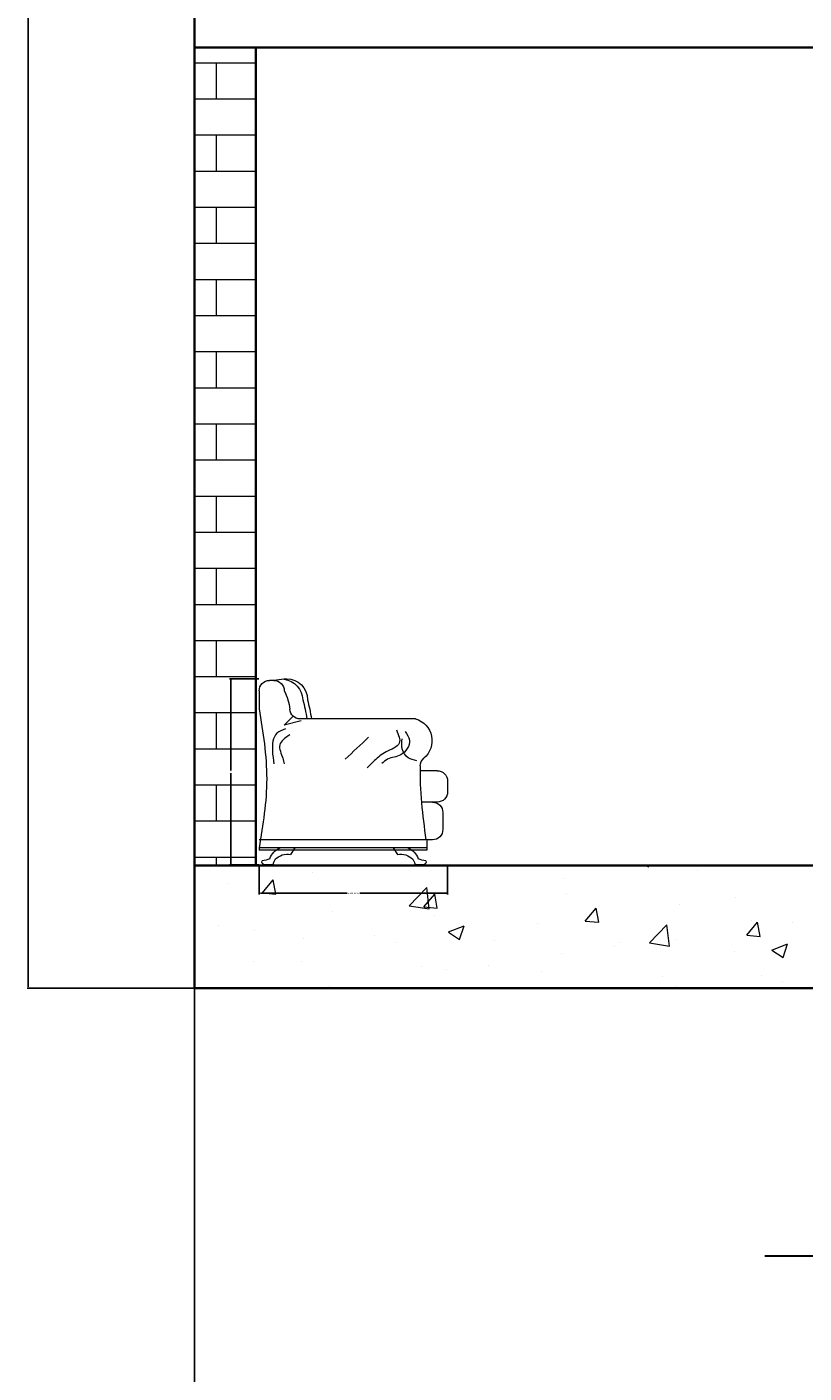
# Model space of a CAD drawing. Units: inches. Extents: x 2416 to 3391, y 1375 to 2496.
# Tile 5 of 13: x 2880 to 2994, y 2069 to 2267. Entities that reach past the tile are written whole.
import ezdxf

# ---------------------------------------------------------------- set-up
doc = ezdxf.new("R2010")
doc.units = ezdxf.units.IN
for name, color, linetype, lineweight in [('A-ANNO-DIMS', 2, 'Continuous', 18), ('A-ANNO-TITL', 7, 'Continuous', 30), ('A-FLOR-PATT', 252, 'Continuous', 13), ('A-FURN', 8, 'Continuous', 18), ('A-SECT', 7, 'Continuous', 35), ('A-WALL-PATT', 252, 'Continuous', 13)]:
    doc.layers.add(name, color=color, linetype=linetype, lineweight=lineweight)
doc.styles.get("Standard").update_dxf_attribs({"font": 'arial.ttf'})
doc.dimstyles.get("Standard").update_dxf_attribs({"dimtxt": 0.18, "dimasz": 0.18, "dimexe": 0.18, "dimexo": 0.0625, "dimgap": 0.09, "dimtad": 0, "dimtih": 1, "dimtoh": 1, "dimdec": 4, "dimzin": 0, "dimdsep": 46, "dimtxsty": 'Standard', "dimcen": 0.09, "dimadec": 0, "dimazin": 0, "dimtfac": 1, "dimtdec": 4, "dimtofl": 0, "dimtmove": 0, "dimatfit": 3, "dimfxl": 1, "dimtolj": 1, "dimtzin": 0, "dimarcsym": 0})

# ---------------------------------------------------------------- blocks, each defined once
blk = doc.blocks.new('A$C624B6646')
for p, q in [((768.9, 888.9), (830, 881)), ((830, 881), (850, 881)), ((900, 831), (900, 744.9)), ((738.1, 710.5), (780, 667.9)), ((153, 697.4), (704.3, 697.4)), ((161, 698), (700, 698)), ((700, 688.2), (780, 667.9)), ((50, 450), (131.5, 450)), ((0, 400), (0, 350)), ((50, 300), (125, 300)), ((22.9, 250), (22.9, 170)), ((72.9, 120), (100, 120)), ((100, 120), (100, 82)), ((100, 82), (900, 82)), ((100, 82), (100, 70)), ((100, 70), (900, 70)), ((104.3, 120.1), (900, 120.1)), ((260.4, 82), (239.5, 50)), ((729.1, 82), (750.1, 50)), ((900, 82), (900, 70)), ((113.5, 1), (155.7, 0)), ((157.5, 12), (155.7, 0)), ((166.5, 27), (157.5, 12)), ((823.1, 27), (832.1, 12)), ((832.1, 12), (833.9, 0)), ((833.9, 0), (876.1, 1))]:
    blk.add_line(p, q)
for centre, radius, start, end in [((768.9, 788.9), 100, 90, 180), ((798.7, 781.1), 107.9, 99.75349, 175.837), ((830, 831), 50, 90, 180), ((850, 831), 50, 0, 90), ((1468.2, 575.1), 826.9, 165.01373, 171.49796), ((1489.9, 575.1), 826.9, 165.01373, 171.49796), ((983.5, 723.2), 230.2, 152.1091, 175.06533), ((704.3, 747.4), 50, 270, 355.06533), ((183.4, 592.9), 108.8, 106.20534, 229.88001), ((50, 400), 50, 90, 180), ((81, 471.5), 50, 1.79104, 49.88001), ((50, 350), 50, 180, 270), ((72.9, 250), 50, 90, 180), ((72.9, 170), 50, 180, 270), ((229.5, -3.6), 95.2, 115.89455, 159.31204), ((760, -3.6), 95.2, 20.68796, 64.10545), ((118.3, 15.7), 15.5, 163.76363, 251.75345), ((97, 117.6), 97.9, 273.83102, 296.417), ((224.1, -28.4), 79.9, 78.85513, 136.12087), ((765.5, -28.4), 79.9, 43.87913, 101.14487), ((892.6, 117.6), 97.9, 243.583, 266.16898), ((871.2, 15.7), 15.5, 288.24655, 16.23637)]:
    blk.add_arc(centre, radius, start, end)
for points, knots in [([(900, 744.9), (881.9, 633.6), (846, 412.5), (882.1, 191.6), (900, 82)], [0, 0, 0, 0, 336.072717, 666.841786, 666.841786, 666.841786, 666.841786]), ([(245, 644.3), (234.7, 621.1), (212.4, 570.7), (298.1, 543.4), (345, 503.6), (373, 474.9), (384.6, 463.1)], [0, 0, 0, 0, 64.284597, 139.770948, 209.553279, 258.887454, 258.887454, 258.887454, 258.887454]), ([(773.7, 649.5), (789.3, 644.1), (833.7, 628.7), (839.7, 550.2), (832.6, 502.4), (829.5, 482.2)], [0, 0, 0, 0, 46.821513, 133.069671, 196.206665, 196.206665, 196.206665, 196.206665]), ([(147.3, 497.9), (162.1, 500.8), (194, 507), (222.9, 552.8), (219, 586.1), (217.1, 602.5)], [0, 0, 0, 0, 44.149611, 94.447762, 143.253115, 143.253115, 143.253115, 143.253115]), ([(203.1, 637.4), (193.5, 623.9), (167.4, 587), (215.6, 514.8), (280.1, 514.7), (305.9, 491.8), (314.8, 484)], [0, 0, 0, 0, 46.783568, 128.12179, 194.346234, 229.237423, 229.237423, 229.237423, 229.237423]), ([(752.7, 621.6), (775, 607.1), (817.9, 579.1), (789.2, 521.1), (782.7, 491.4), (780.7, 482.2)], [0, 0, 0, 0, 69.067804, 133.352323, 162.101735, 162.101735, 162.101735, 162.101735])]:
    blk.add_open_spline(points, degree=3, knots=knots)
for points in [[(377.6, 609.5), (414.9, 574.6), (452.1, 539.7), (489.4, 504.9)], [(131, 473), (134.7, 356.2), (119.5, 238.2), (104.3, 120.1)]]:
    blk.add_open_spline(points, degree=3)
blk = doc.blocks.new('A$C4C705FAE')
blk.add_blockref('A$C624B6646', (0, 0))
blk = doc.blocks.new('*D43')
at = {"layer": 'A-ANNO-DIMS', "color": 0, "lineweight": -2, "transparency": 16777216}
for p, q in [((2913.66, 2143.87), (2913.66, 2139.6)), ((2941.32, 2143.87), (2941.32, 2139.6)), ((2913.84, 2139.78), (2926.56, 2139.78)), ((2941.14, 2139.78), (2928.42, 2139.78))]:
    blk.add_line(p, q, dxfattribs=at)
at = {"layer": 'A-ANNO-DIMS', "color": 0, "transparency": 16777216}
for points in [[(2913.84, 2139.81), (2913.84, 2139.75), (2913.66, 2139.78)], [(2941.14, 2139.81), (2941.14, 2139.75), (2941.32, 2139.78)]]:
    blk.add_solid(points, dxfattribs=at)
at = {"layer": 'Defpoints', "color": 0, "transparency": 16777216}
for p in [(2913.66, 2143.93), (2941.32, 2143.93), (2913.66, 2139.78)]:
    blk.add_point(p, dxfattribs=at)
at = {"layer": 'A-ANNO-DIMS', "color": 0, "transparency": 16777216, "insert": (2927.49, 2139.78), "char_height": 0.18, "attachment_point": 5}
blk.add_mtext('\\A1;ARMCHAIR 28', dxfattribs=at)
blk = doc.blocks.new('*D44')
at = {"layer": 'A-ANNO-DIMS', "color": 0, "lineweight": -2, "transparency": 16777216}
for p, q in [((2913.6, 2171.25), (2909.33, 2171.25)), ((2909.51, 2171.07), (2909.51, 2157.77)), ((2909.51, 2144.11), (2909.51, 2157.41)), ((2913.6, 2143.93), (2909.33, 2143.93))]:
    blk.add_line(p, q, dxfattribs=at)
at = {"layer": 'A-ANNO-DIMS', "color": 0, "transparency": 16777216}
for points in [[(2909.48, 2171.07), (2909.54, 2171.07), (2909.51, 2171.25)], [(2909.48, 2144.11), (2909.54, 2144.11), (2909.51, 2143.93)]]:
    blk.add_solid(points, dxfattribs=at)
at = {"layer": 'Defpoints', "color": 0, "transparency": 16777216}
for p in [(2909.51, 2171.25), (2913.66, 2171.25), (2913.66, 2143.93)]:
    blk.add_point(p, dxfattribs=at)
at = {"layer": 'A-ANNO-DIMS', "color": 0, "transparency": 16777216, "insert": (2909.51, 2157.59), "char_height": 0.18, "attachment_point": 5}
blk.add_mtext('\\A1;27', dxfattribs=at)
blk = doc.blocks.new('*D83')
at = {"layer": 'A-ANNO-DIMS', "color": 0, "lineweight": -2, "transparency": 16777216}
for p, q in [((2904.19, 2125.8), (2904.19, 2062.03)), ((3202.69, 2125.8), (3202.69, 2062.03)), ((2904.37, 2062.21), (3053.05, 2062.21)), ((3202.51, 2062.21), (3053.84, 2062.21))]:
    blk.add_line(p, q, dxfattribs=at)
at = {"layer": 'A-ANNO-DIMS', "color": 0, "transparency": 16777216}
for points in [[(2904.37, 2062.24), (2904.37, 2062.18), (2904.19, 2062.21)], [(3202.51, 2062.24), (3202.51, 2062.18), (3202.69, 2062.21)]]:
    blk.add_solid(points, dxfattribs=at)
at = {"layer": 'Defpoints', "color": 0, "transparency": 16777216}
for p in [(2904.19, 2125.86), (3202.69, 2125.86), (3202.69, 2062.21)]:
    blk.add_point(p, dxfattribs=at)
at = {"layer": 'A-ANNO-DIMS', "color": 0, "transparency": 16777216, "insert": (3053.44, 2062.21), "char_height": 0.18, "attachment_point": 5}
blk.add_mtext('\\A1;298.5', dxfattribs=at)
blk = doc.blocks.new('*D84')
at = {"layer": 'A-ANNO-DIMS', "color": 0, "lineweight": -2, "transparency": 16777216}
for p, q in [((2904.13, 2437.86), (2879.61, 2437.86)), ((2879.79, 2437.68), (2879.79, 2282.04)), ((2879.79, 2126.04), (2879.79, 2281.68)), ((2904.13, 2125.86), (2879.61, 2125.86))]:
    blk.add_line(p, q, dxfattribs=at)
at = {"layer": 'A-ANNO-DIMS', "color": 0, "transparency": 16777216}
for points in [[(2879.76, 2437.68), (2879.82, 2437.68), (2879.79, 2437.86)], [(2879.76, 2126.04), (2879.82, 2126.04), (2879.79, 2125.86)]]:
    blk.add_solid(points, dxfattribs=at)
at = {"layer": 'Defpoints', "color": 0, "transparency": 16777216}
for p in [(2879.79, 2437.86), (2904.19, 2437.86), (2904.19, 2125.86)]:
    blk.add_point(p, dxfattribs=at)
at = {"layer": 'A-ANNO-DIMS', "color": 0, "transparency": 16777216, "insert": (2879.79, 2281.86), "char_height": 0.18, "attachment_point": 5}
blk.add_mtext('\\A1;312', dxfattribs=at)

msp = doc.modelspace()

# ---------------------------------------------------------------- hatches: boundary and pattern name
at = {"layer": 'A-FLOR-PATT'}
h = msp.add_hatch(dxfattribs=at)
h.set_pattern_fill('AR-CONC', color=256, scale=0.13, style=0)
h.paths.add_polyline_path([(2904.1924, 2125.8608), (3202.6924, 2125.8608), (3202.6924, 2143.8608), (2904.1924, 2143.8608)])
at = {"layer": 'A-WALL-PATT'}
h = msp.add_hatch(dxfattribs=at)
h.set_pattern_fill('AR-BRSTD', color=256, scale=0.0781866, style=0)
h.paths.add_polyline_path([(2904.1924, 2143.8608), (2913.1924, 2143.8608), (2913.1924, 2263.8608), (2904.1924, 2263.8608)])

# ---------------------------------------------------------------- linework, layer by layer
at = {"layer": 'A-ANNO-TITL'}
msp.add_line((2987.8706, 2086.6125), (3103.051, 2086.6125), dxfattribs=at)
at = {"layer": 'A-SECT'}
for p, q in [((2904.1924, 2437.8608), (2904.1924, 2251.8608)), ((2904.1924, 2311.8608), (2904.1924, 2125.8608)), ((3202.6924, 2263.8608), (2904.1924, 2263.8608)), ((2913.1924, 2263.8608), (2913.1924, 2143.8608)), ((3202.6924, 2143.8608), (2904.1924, 2143.8608)), ((3202.6924, 2125.8608), (2904.1924, 2125.8608))]:
    msp.add_line(p, q, dxfattribs=at)

# ---------------------------------------------------------------- block references
at = {"layer": 'A-FURN', "xscale": -0.0307315214408566, "yscale": 0.0307315214408566, "zscale": 0.0307315214408566}
msp.add_blockref('A$C4C705FAE', (2941.3184, 2143.9311), dxfattribs=at)

# ---------------------------------------------------------------- dimensions: what is measured, and where the dimension line sits
at = {"layer": 'A-ANNO-DIMS'}
for base, p1, p2, picture, middle in [((2879.7924, 2437.8608), (2904.1924, 2125.8608), (2904.1924, 2437.8608), '*D84', (2879.7924, 2281.8608)), ((2909.5113, 2171.2493), (2913.66, 2143.9311), (2913.66, 2171.2493), '*D44', (2909.5113, 2157.5902))]:
    dim = msp.add_linear_dim(base=base, p1=p1, p2=p2, angle=90, dimstyle='Standard', override={"dimdec": 0, "dimlfac": 1, "dimrnd": 0, "dimzin": 0, "dimdsep": 46, "dimlunit": 2}, dxfattribs=at)
    dim.commit()
    dim.dimension.update_dxf_attribs({"geometry": picture, "text_midpoint": middle})
dim = msp.add_linear_dim(base=(2913.66, 2139.7824), p1=(2941.3184, 2143.9311), p2=(2913.66, 2143.9311), angle=180, text='ARMCHAIR <>', dimstyle='Standard', override={"dimdec": 0, "dimlfac": 1, "dimrnd": 0, "dimzin": 0, "dimdsep": 46, "dimlunit": 2}, dxfattribs=at)
dim.commit()
dim.dimension.update_dxf_attribs({"geometry": '*D43', "text_midpoint": (2927.4892, 2139.7824)})
dim = msp.add_linear_dim(base=(3202.6924, 2062.2125), p1=(2904.1924, 2125.8608), p2=(3202.6924, 2125.8608), dimstyle='Standard', override={"dimdec": 1, "dimlfac": 1, "dimrnd": 0, "dimzin": 0, "dimdsep": 46, "dimlunit": 2}, dxfattribs=at)
dim.commit()
dim.dimension.update_dxf_attribs({"geometry": '*D83', "text_midpoint": (3053.4424, 2062.2125)})

doc.saveas('drawing.dxf')
